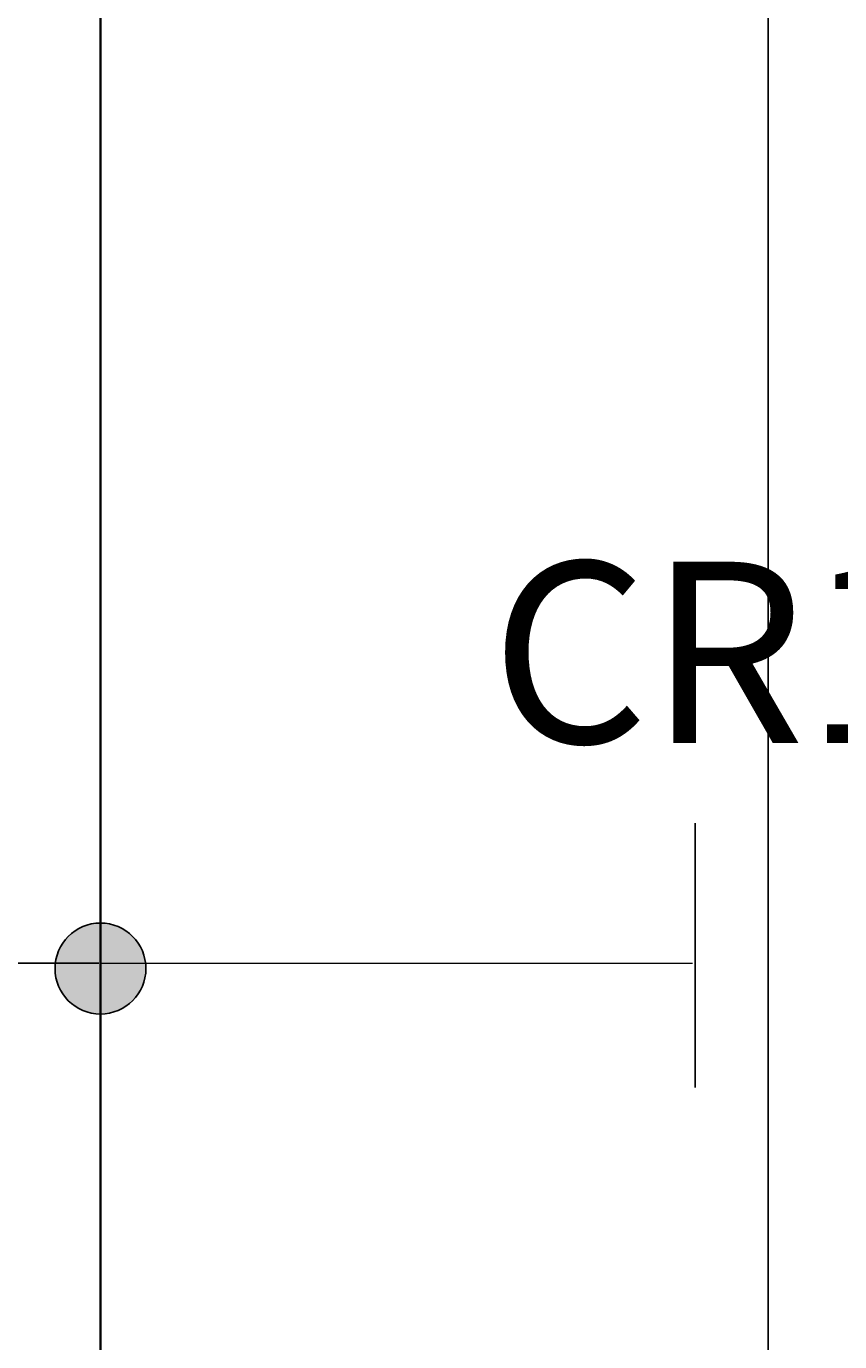
# Model space of a CAD drawing. Units: inches. Extents: x 738 to 1068, y 378 to 757.
# Tile 9 of 41: x 779 to 806, y 449 to 492. Entities that reach past the tile are written whole.
import ezdxf

# ---------------------------------------------------------------- set-up
doc = ezdxf.new("R2010")
doc.units = ezdxf.units.IN
doc.header["$MEASUREMENT"] = 0
for name, color, linetype, lineweight in [('A-ANNO-DIMS', 2, 'Continuous', 18), ('E-ANNO-TEXT', 7, 'Continuous', 18), ('E-CONN', 7, 'Continuous', 25), ('E-CTRL-CONT', 4, 'Continuous', 25), ('E-CTRL-WIRE', 7, 'Continuous', 18), ('E-POWR-FEED', 7, 'Continuous', 35)]:
    doc.layers.add(name, color=color, linetype=linetype, lineweight=lineweight)
doc.styles.get("Standard").update_dxf_attribs({"font": 'arial.ttf'})
doc.dimstyles.get("Standard").update_dxf_attribs({"dimtxt": 0.18, "dimasz": 0.18, "dimexe": 0.18, "dimexo": 0.0625, "dimgap": 0.09, "dimtad": 0, "dimtih": 1, "dimtoh": 1, "dimdec": 4, "dimzin": 0, "dimdsep": 46, "dimtxsty": 'Standard', "dimcen": 0.09, "dimadec": 0, "dimazin": 0, "dimtfac": 1, "dimtdec": 4, "dimtofl": 0, "dimtmove": 0, "dimatfit": 3, "dimfxl": 1, "dimtolj": 1, "dimtzin": 0, "dimarcsym": 0})

# ---------------------------------------------------------------- blocks, each defined once
blk = doc.blocks.new('CR-AUX-CONTACT-NO')
for p, q in [((0, 8.72), (0, 0)), ((8.265, 8.72), (8.265, 0))]:
    blk.add_line(p, q)
blk = doc.blocks.new('RUNG-JUNCTION')
h = blk.add_hatch(color=256)
h.dxf.hatch_style = 1
h.paths.add_polyline_path([(3, 1.5, 1), (0, 1.5, 1)])
blk.add_lwpolyline([(0, 1.5, 1), (3, 1.5, 1)], format="xyb", close=True)
blk = doc.blocks.new('*D20')
at = {"layer": 'A-ANNO-DIMS', "color": 0, "lineweight": -2, "transparency": 16777216}
for p, q in [((781.427, 461.392), (738.194, 461.392)), ((738.374, 461.212), (738.374, 454.01)), ((738.374, 446.445), (738.374, 453.647)), ((781.422, 446.265), (738.194, 446.265))]:
    blk.add_line(p, q, dxfattribs=at)
at = {"layer": 'A-ANNO-DIMS', "color": 0, "transparency": 16777216}
for points in [[(738.344, 461.212), (738.404, 461.212), (738.374, 461.392)], [(738.344, 446.445), (738.404, 446.445), (738.374, 446.265)]]:
    blk.add_solid(points, dxfattribs=at)
at = {"layer": 'Defpoints', "color": 0, "transparency": 16777216}
for p in [(738.374, 461.392), (781.49, 461.392), (781.485, 446.265)]:
    blk.add_point(p, dxfattribs=at)
at = {"layer": 'A-ANNO-DIMS', "color": 0, "transparency": 16777216, "insert": (738.374, 453.829), "char_height": 0.18, "attachment_point": 5}
blk.add_mtext('\\A1;15.127', dxfattribs=at)
blk = doc.blocks.new('*D21')
at = {"layer": 'A-ANNO-DIMS', "color": 0, "lineweight": -2, "transparency": 16777216}
for p, q in [((781.427, 531.401), (738.194, 531.401)), ((738.374, 531.221), (738.374, 496.578)), ((738.374, 461.572), (738.374, 496.215)), ((781.427, 461.392), (738.194, 461.392))]:
    blk.add_line(p, q, dxfattribs=at)
at = {"layer": 'A-ANNO-DIMS', "color": 0, "transparency": 16777216}
for points in [[(738.344, 531.221), (738.404, 531.221), (738.374, 531.401)], [(738.344, 461.572), (738.404, 461.572), (738.374, 461.392)]]:
    blk.add_solid(points, dxfattribs=at)
at = {"layer": 'Defpoints', "color": 0, "transparency": 16777216}
for p in [(738.374, 531.401), (781.49, 531.401), (781.49, 461.392)]:
    blk.add_point(p, dxfattribs=at)
at = {"layer": 'A-ANNO-DIMS', "color": 0, "transparency": 16777216, "insert": (738.374, 496.396), "char_height": 0.18, "attachment_point": 5}
blk.add_mtext('\\A1;70.01', dxfattribs=at)
blk = doc.blocks.new('*D25')
at = {"layer": 'A-ANNO-DIMS', "color": 0, "lineweight": -2, "transparency": 16777216}
for p, q in [((781.49, 646.923), (781.49, 378.239)), ((803.522, 646.923), (803.522, 378.239)), ((781.67, 378.419), (792.111, 378.419)), ((803.342, 378.419), (792.901, 378.419))]:
    blk.add_line(p, q, dxfattribs=at)
at = {"layer": 'A-ANNO-DIMS', "color": 0, "transparency": 16777216}
for points in [[(781.67, 378.449), (781.67, 378.389), (781.49, 378.419)], [(803.342, 378.449), (803.342, 378.389), (803.522, 378.419)]]:
    blk.add_solid(points, dxfattribs=at)
at = {"layer": 'Defpoints', "color": 0, "transparency": 16777216}
for p in [(781.49, 646.985), (803.522, 646.985), (803.522, 378.419)]:
    blk.add_point(p, dxfattribs=at)
at = {"layer": 'A-ANNO-DIMS', "color": 0, "transparency": 16777216, "insert": (792.506, 378.419), "char_height": 0.18, "attachment_point": 5}
blk.add_mtext('\\A1;22.03', dxfattribs=at)
blk = doc.blocks.new('*D34')
at = {"layer": 'A-ANNO-DIMS', "color": 0, "lineweight": -2, "transparency": 16777216}
for p, q in [((781.49, 686.266), (781.49, 378.239)), ((830.489, 686.266), (830.489, 378.239)), ((781.67, 378.419), (805.767, 378.419)), ((830.309, 378.419), (806.212, 378.419))]:
    blk.add_line(p, q, dxfattribs=at)
at = {"layer": 'A-ANNO-DIMS', "color": 0, "transparency": 16777216}
for points in [[(781.67, 378.449), (781.67, 378.389), (781.49, 378.419)], [(830.309, 378.449), (830.309, 378.389), (830.489, 378.419)]]:
    blk.add_solid(points, dxfattribs=at)
at = {"layer": 'Defpoints', "color": 0, "transparency": 16777216}
for p in [(781.49, 686.329), (830.489, 686.329), (830.489, 378.419)]:
    blk.add_point(p, dxfattribs=at)
at = {"layer": 'A-ANNO-DIMS', "color": 0, "transparency": 16777216, "insert": (805.99, 378.419), "char_height": 0.18, "attachment_point": 5}
blk.add_mtext('\\A1;49', dxfattribs=at)
blk = doc.blocks.new('*D38')
at = {"layer": 'A-ANNO-DIMS', "color": 0, "lineweight": -2, "transparency": 16777216}
for p, q in [((781.485, 593.017), (781.485, 378.239)), ((887.04, 593.067), (887.04, 378.239)), ((781.665, 378.419), (833.807, 378.419)), ((886.86, 378.419), (834.718, 378.419))]:
    blk.add_line(p, q, dxfattribs=at)
at = {"layer": 'A-ANNO-DIMS', "color": 0, "transparency": 16777216}
for points in [[(781.665, 378.449), (781.665, 378.389), (781.485, 378.419)], [(886.86, 378.449), (886.86, 378.389), (887.04, 378.419)]]:
    blk.add_solid(points, dxfattribs=at)
at = {"layer": 'Defpoints', "color": 0, "transparency": 16777216}
for p in [(887.04, 593.13), (781.485, 593.08), (887.04, 378.419)]:
    blk.add_point(p, dxfattribs=at)
at = {"layer": 'A-ANNO-DIMS', "color": 0, "transparency": 16777216, "insert": (834.263, 378.419), "char_height": 0.18, "attachment_point": 5}
blk.add_mtext('\\A1;105.56', dxfattribs=at)

msp = doc.modelspace()

# ---------------------------------------------------------------- linework, layer by layer
at = {"layer": 'E-CTRL-WIRE'}
msp.add_line((781.4897, 461.3919), (801.0218, 461.3919), dxfattribs=at)
at = {"layer": 'E-POWR-FEED'}
msp.add_line((781.4897, 686.329), (781.4897, 437.7164), dxfattribs=at)

# ---------------------------------------------------------------- block references
at = {"layer": 'E-CONN'}
msp.add_blockref('RUNG-JUNCTION', (779.985, 459.7136), dxfattribs=at)
at = {"layer": 'E-CTRL-CONT'}
msp.add_blockref('CR-AUX-CONTACT-NO', (801.115, 457.29), dxfattribs=at)

# ---------------------------------------------------------------- texts
at = {"layer": 'E-ANNO-TEXT'}
msp.add_text('CR1-3', height=5.97842, dxfattribs=at).set_placement((794.3655, 468.6537))

# ---------------------------------------------------------------- dimensions: what is measured, and where the dimension line sits
at = {"layer": 'A-ANNO-DIMS'}
for base, p1, p2, override, picture, middle in [((830.4893, 378.4191), (781.4897, 686.329), (830.4893, 686.329), {"dimdec": 0, "dimlfac": 1, "dimrnd": 0, "dimzin": 0, "dimdsep": 46, "dimlunit": 2}, '*D34', (805.9895, 378.4191)), ((803.5218, 378.4191), (781.4897, 646.9853), (803.5218, 646.9853), {"dimdec": 2, "dimlfac": 1, "dimrnd": 0, "dimzin": 0, "dimdsep": 46, "dimlunit": 2}, '*D25', (792.5057, 378.4191)), ((887.0404, 378.4191), (781.4846, 593.0796), (887.0404, 593.1296), {"dimdec": 2, "dimlfac": 1, "dimrnd": 0, "dimzin": 0, "dimdsep": 46, "dimlunit": 2}, '*D38', (834.2625, 378.4191))]:
    dim = msp.add_linear_dim(base=base, p1=p1, p2=p2, dimstyle='Standard', override=override, dxfattribs=at)
    dim.commit()
    dim.dimension.update_dxf_attribs({"geometry": picture, "text_midpoint": middle})
for base, p1, p2, override, picture, middle in [((738.3736, 531.4009), (781.4897, 461.3919), (781.4897, 531.4009), {"dimdec": 2, "dimlfac": 1, "dimrnd": 0, "dimzin": 0, "dimdsep": 46, "dimlunit": 2}, '*D21', (738.3736, 496.3964)), ((738.3736, 461.3919), (781.4846, 446.2651), (781.4897, 461.3919), {"dimdec": 3, "dimlfac": 1, "dimrnd": 0, "dimzin": 0, "dimdsep": 46, "dimlunit": 2}, '*D20', (738.3736, 453.8285))]:
    dim = msp.add_linear_dim(base=base, p1=p1, p2=p2, angle=90, dimstyle='Standard', override=override, dxfattribs=at)
    dim.commit()
    dim.dimension.update_dxf_attribs({"geometry": picture, "text_midpoint": middle})

doc.saveas('drawing.dxf')
